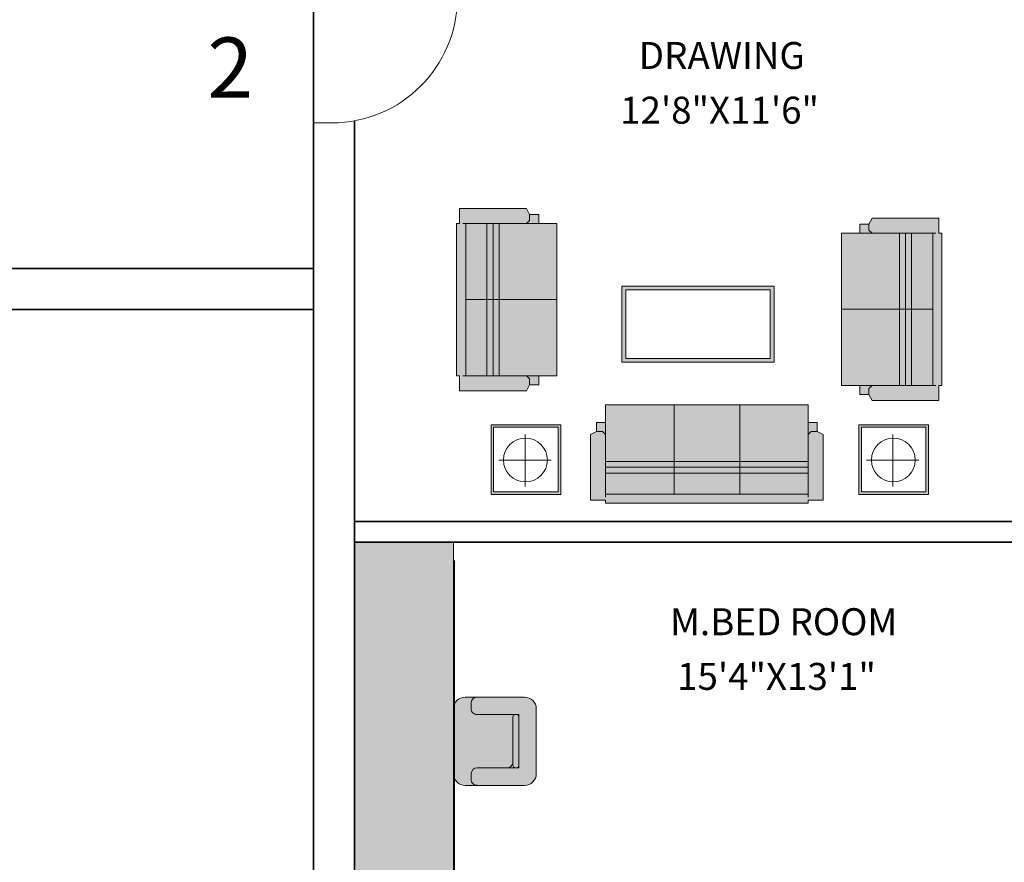
# Model space of a CAD drawing. Units: millimetres. Extents: x 27017497 to 27018854, y 7058029 to 7059154.
# Tile 78 of 91: x 27018246 to 27018462, y 7058224 to 7058409. Entities that reach past the tile are written whole.
import ezdxf

# ---------------------------------------------------------------- set-up
doc = ezdxf.new("R2010")
doc.units = ezdxf.units.MM
for name, color, linetype, lineweight in [('A-ANNO-DIMS', 2, 'Continuous', 18), ('A-ANNO-IDEN', 7, 'Continuous', 18), ('A-AREA-IDEN', 7, 'Continuous', 18), ('A-DOOR', 4, 'Continuous', 20), ('A-FLOR-CASE', 8, 'Continuous', 20), ('A-FLOR-CASE-PATT', 44, 'Continuous', 13), ('A-FURN', 8, 'Continuous', 18), ('A-WALL', 7, 'Continuous', 35)]:
    doc.layers.add(name, color=color, linetype=linetype, lineweight=lineweight)
doc.layers.add('A-FURN-PATT', color=177, linetype='Continuous', lineweight=13, true_color=0x293189)
doc.styles.get("Standard").update_dxf_attribs({"font": 'arial.ttf'})
doc.dimstyles.get("Standard").update_dxf_attribs({"dimtxt": 0.18, "dimasz": 0.18, "dimexe": 0.18, "dimexo": 0.0625, "dimgap": 0.09, "dimtad": 0, "dimtih": 1, "dimtoh": 1, "dimdec": 4, "dimzin": 0, "dimdsep": 46, "dimtxsty": 'Standard', "dimcen": 0.09, "dimadec": 0, "dimazin": 0, "dimtfac": 1, "dimtdec": 4, "dimtofl": 0, "dimtmove": 0, "dimatfit": 3, "dimfxl": 1, "dimtolj": 1, "dimtzin": 0, "dimarcsym": 0})

# ---------------------------------------------------------------- blocks, each defined once
blk = doc.blocks.new('*U2')
for p, q in [((0, 0), (0, -6)), ((40, 0), (40, -6))]:
    blk.add_line(p, q)
blk.add_lwpolyline([(0, 0), (0, 40), (1.75, 40), (1.75, 0)], close=True)
blk.add_arc((0, 0), 40, 0, 90)
blk = doc.blocks.new('CHAIR-OCCASIONAL')
for p, q in [((19.6, 18.74), (7.02, 22.21)), ((3.87, 20.42), (0.09, 6.71)), ((4.13, 6.92), (7.23, 18.17)), ((5.25, 10.97), (7.23, 18.17)), ((5.25, 10.97), (7.1, 17.68)), ((8.33, 17.34), (5.63, 7.52)), ((16.06, 15.73), (7.23, 18.17)), ((7.23, 18.17), (16.06, 15.73)), ((7.23, 18.17), (16.06, 15.73)), ((7.73, 18.03), (7.97, 17.97)), ((7.73, 18.03), (7.97, 17.97)), ((17.64, 16.63), (17.98, 17.86)), ((17.64, 16.63), (17.98, 17.86)), ((17.6, 1.88), (21.39, 15.6)), ((12.96, 4.48), (4.13, 6.92)), ((4.87, 6.71), (4.63, 6.78)), ((5.63, 7.52), (5.5, 7.07)), ((1.88, 3.56), (14.46, 0.09)), ((13.86, 2.91), (13.52, 1.68))]:
    blk.add_line(p, q)
for centre, radius, start, end in [((6.34, 19.74), 2.56, 74.5879, 164.5879), ((16.74, 18.2), 1.28, 344.5879, 74.5879), ((16.74, 18.2), 1.28, 344.5879, 74.5879), ((7.59, 17.54), 0.512, 74.5879, 164.5879), ((7.84, 17.47), 0.512, 344.5879, 74.5879), ((9.36, 16.26), 1.28, 74.5879, 164.5879), ((18.92, 16.28), 2.56, 344.5879, 74.5879), ((16.4, 16.97), 1.28, 254.5879, 344.5879), ((16.4, 16.97), 1.28, 254.5879, 344.5879), ((2.56, 6.03), 2.56, 164.5879, 254.5879), ((4.76, 7.28), 0.512, 164.5879, 254.5879), ((5.01, 7.21), 0.512, 254.5879, 344.5879), ((12.62, 3.25), 1.28, 344.5879, 74.5879), ((12.28, 2.02), 1.28, 254.5879, 344.5879), ((15.14, 2.56), 2.56, 254.5879, 344.5879)]:
    blk.add_arc(centre, radius, start, end)
blk = doc.blocks.new('SOFA-THREE-SEAT')
for p, q in [((47.73, 21.58), (3.27, 21.58)), ((3.27, 21.58), (3.27, 17.65)), ((18.31, 21.58), (18.31, 1.96)), ((32.69, 21.58), (32.69, 1.96)), ((47.73, 17.65), (47.73, 21.58)), ((3.27, 17.65), (1.31, 17.65)), ((1.31, 17.65), (1.31, 15.69)), ((3.27, 17.65), (3.27, 15.04)), ((47.73, 17.65), (47.73, 15.04)), ((49.69, 17.65), (47.73, 17.65)), ((49.69, 15.69), (49.69, 17.65)), ((1.31, 15.69), (0, 15.04)), ((1.31, 15.69), (2.62, 15.69)), ((2.62, 15.69), (3.27, 15.04)), ((48.38, 15.69), (47.73, 15.04)), ((49.69, 15.69), (48.38, 15.69)), ((51, 15.04), (49.69, 15.69)), ((0, 15.04), (0, 0.65)), ((3.27, 15.04), (3.27, 1.31)), ((47.73, 15.04), (47.73, 1.31)), ((51, 0.65), (51, 15.04)), ((47.73, 9.15), (3.27, 9.15)), ((47.73, 7.85), (3.27, 7.85)), ((47.73, 6.54), (3.27, 6.54)), ((0, 0.65), (3.27, 0.65)), ((3.27, 1.96), (47.73, 1.96)), ((3.27, 0.65), (3.27, 0)), ((47.73, 0), (47.73, 0.65)), ((47.73, 0.65), (51, 0.65)), ((3.27, 0), (47.73, 0))]:
    blk.add_line(p, q)
blk = doc.blocks.new('SETTEE-TWO-SEAT')
for p, q in [((6.67, 40.01), (6, 38.68)), ((21.34, 40.01), (6.67, 40.01)), ((21.34, 36.68), (21.34, 40.01)), ((6, 38.68), (4, 38.68)), ((4, 38.68), (4, 36.68)), ((6, 38.68), (6, 37.35)), ((6, 37.35), (6.67, 36.68)), ((0, 36.68), (0, 3.33)), ((4, 36.68), (0, 36.68)), ((4, 36.68), (6.67, 36.68)), ((6.67, 36.68), (20.67, 36.68)), ((12.67, 36.68), (12.67, 3.33)), ((14, 36.68), (14, 3.33)), ((15.34, 36.68), (15.34, 3.33)), ((20.01, 3.33), (20.01, 36.68)), ((22.01, 36.68), (21.34, 36.68)), ((22.01, 3.33), (22.01, 36.68)), ((0, 20.01), (20.01, 20.01)), ((0, 3.33), (4, 3.33)), ((4, 3.33), (6.67, 3.33)), ((4, 3.33), (4, 1.33)), ((6, 2.67), (6.67, 3.33)), ((6, 1.33), (6, 2.67)), ((6.67, 3.33), (20.67, 3.33)), ((21.34, 0), (21.34, 3.33)), ((21.34, 3.33), (22.01, 3.33)), ((4, 1.33), (6, 1.33)), ((6, 1.33), (6.67, 0)), ((6.67, 0), (21.34, 0))]:
    blk.add_line(p, q)
blk = doc.blocks.new('TABLE-END')
for p, q in [((15.28, 15.28), (0, 15.28)), ((0, 15.28), (0, 0)), ((15.28, 0), (15.28, 15.28)), ((14.73, 14.73), (0.56, 14.73)), ((0.56, 14.73), (0.56, 0.56)), ((7.79, 1.78), (7.79, 13.18)), ((14.73, 0.56), (14.73, 14.73)), ((2.12, 7.51), (13.57, 7.51)), ((0.56, 0.56), (14.73, 0.56)), ((0, 0), (15.28, 0))]:
    blk.add_line(p, q)
blk.add_circle((7.72, 7.57), 4.81)
blk = doc.blocks.new('TABLE-COFFEE')
for p, q in [((33.35, 16.67), (0, 16.67)), ((0, 16.67), (0, 0)), ((32.51, 15.84), (0.83, 15.84)), ((0.83, 15.84), (0.83, 0.83)), ((32.51, 0.83), (32.51, 15.84)), ((33.35, 0), (33.35, 16.67)), ((0, 0), (33.35, 0)), ((0.83, 0.83), (32.51, 0.83))]:
    blk.add_line(p, q)
blk = doc.blocks.new('*D47')
at = {"layer": 'A-ANNO-DIMS', "color": 0, "lineweight": -2, "transparency": 16777216}
for p, q in [((27017561.17, 7058294.35), (27017561.17, 7058028.6)), ((27018790.61, 7058294.35), (27018790.61, 7058028.6)), ((27017561.35, 7058028.78), (27018175.43, 7058028.78)), ((27018790.43, 7058028.78), (27018176.34, 7058028.78))]:
    blk.add_line(p, q, dxfattribs=at)
at = {"layer": 'A-ANNO-DIMS', "color": 0, "transparency": 16777216}
for points in [[(27017561.35, 7058028.81), (27017561.35, 7058028.75), (27017561.17, 7058028.78)], [(27018790.43, 7058028.81), (27018790.43, 7058028.75), (27018790.61, 7058028.78)]]:
    blk.add_solid(points, dxfattribs=at)
at = {"layer": 'Defpoints', "color": 0, "transparency": 16777216}
for p in [(27017561.17, 7058294.41), (27018790.61, 7058294.41), (27018790.61, 7058028.78)]:
    blk.add_point(p, dxfattribs=at)
at = {"layer": 'A-ANNO-DIMS', "color": 0, "transparency": 16777216, "insert": (27018175.89, 7058028.78), "char_height": 0.18, "attachment_point": 5}
blk.add_mtext('\\A1;1229.4', dxfattribs=at)
blk = doc.blocks.new('*D48')
at = {"layer": 'A-ANNO-DIMS', "color": 0, "lineweight": -2, "transparency": 16777216}
for p, q in [((27018463.5, 7058622.91), (27017497.54, 7058622.91)), ((27017497.72, 7058622.73), (27017497.72, 7058357.75)), ((27017497.72, 7058092.41), (27017497.72, 7058357.39)), ((27018555.13, 7058092.23), (27017497.54, 7058092.23))]:
    blk.add_line(p, q, dxfattribs=at)
at = {"layer": 'A-ANNO-DIMS', "color": 0, "transparency": 16777216}
for points in [[(27017497.69, 7058622.73), (27017497.75, 7058622.73), (27017497.72, 7058622.91)], [(27017497.69, 7058092.41), (27017497.75, 7058092.41), (27017497.72, 7058092.23)]]:
    blk.add_solid(points, dxfattribs=at)
at = {"layer": 'Defpoints', "color": 0, "transparency": 16777216}
for p in [(27018463.56, 7058622.91), (27017497.72, 7058092.23), (27018555.19, 7058092.23)]:
    blk.add_point(p, dxfattribs=at)
at = {"layer": 'A-ANNO-DIMS', "color": 0, "transparency": 16777216, "insert": (27017497.72, 7058357.57), "char_height": 0.18, "attachment_point": 5}
blk.add_mtext('\\A1;530.7', dxfattribs=at)
blk = doc.blocks.new('*D51')
at = {"layer": 'A-ANNO-DIMS', "color": 0, "lineweight": -2, "transparency": 16777216}
for p, q in [((27018041.17, 7058345.35), (27018041.17, 7058028.6)), ((27018310.61, 7058345.35), (27018310.61, 7058028.6)), ((27018041.35, 7058028.78), (27018175.42, 7058028.78)), ((27018310.43, 7058028.78), (27018176.35, 7058028.78))]:
    blk.add_line(p, q, dxfattribs=at)
at = {"layer": 'A-ANNO-DIMS', "color": 0, "transparency": 16777216}
for points in [[(27018041.35, 7058028.81), (27018041.35, 7058028.75), (27018041.17, 7058028.78)], [(27018310.43, 7058028.81), (27018310.43, 7058028.75), (27018310.61, 7058028.78)]]:
    blk.add_solid(points, dxfattribs=at)
at = {"layer": 'Defpoints', "color": 0, "transparency": 16777216}
for p in [(27018041.17, 7058345.41), (27018310.61, 7058345.41), (27018310.61, 7058028.78)]:
    blk.add_point(p, dxfattribs=at)
at = {"layer": 'A-ANNO-DIMS', "color": 0, "transparency": 16777216, "insert": (27018175.89, 7058028.78), "char_height": 0.18, "attachment_point": 5}
blk.add_mtext('\\A1;269.44', dxfattribs=at)

msp = doc.modelspace()

# ---------------------------------------------------------------- hatches: boundary and pattern name
at = {"layer": 'A-FLOR-CASE-PATT'}
h = msp.add_hatch(color=256, dxfattribs=at)
h.dxf.hatch_style = 1
edge = h.paths.add_edge_path()
edge.add_line((27018341.343, 7058207.055), (27018330.837, 7058207.055))
edge.add_line((27018330.837, 7058207.055), (27018330.837, 7058203.02))
edge.add_line((27018330.837, 7058203.02), (27018338.424, 7058203.02))
edge.add_ellipse((27018338.23, 7058202.551), major_axis=(0.528, 0), ratio=0.8888917, start_angle=0, end_angle=90, ccw=False)
edge.add_line((27018338.758, 7058202.551), (27018338.758, 7058202.238))
edge.add_line((27018338.758, 7058202.238), (27018330.837, 7058201.488))
edge.add_line((27018330.837, 7058201.488), (27018330.837, 7058199.747))
edge.add_line((27018330.837, 7058199.747), (27018338.424, 7058199.747))
edge.add_ellipse((27018338.23, 7058199.277), major_axis=(0.528, 0), ratio=0.8888917, start_angle=0, end_angle=90, ccw=False)
edge.add_line((27018338.758, 7058199.277), (27018338.758, 7058198.964))
edge.add_line((27018338.758, 7058198.964), (27018330.837, 7058198.215))
edge.add_line((27018330.837, 7058198.215), (27018330.837, 7058193.415))
edge.add_line((27018330.837, 7058193.415), (27018338.284, 7058190.704))
edge.add_ellipse((27018337.942, 7058190.329), major_axis=(0.496, -0.181), ratio=0.8888917, start_angle=0, end_angle=90, ccw=False)
edge.add_line((27018338.439, 7058190.148), (27018338.331, 7058189.854))
edge.add_line((27018338.331, 7058189.854), (27018330.837, 7058191.806))
edge.add_line((27018330.837, 7058191.806), (27018330.837, 7058188.22))
edge.add_line((27018330.837, 7058188.22), (27018338.424, 7058188.22))
edge.add_ellipse((27018338.23, 7058187.75), major_axis=(0.528, 0), ratio=0.8888917, start_angle=0, end_angle=90, ccw=False)
edge.add_line((27018338.758, 7058187.75), (27018338.758, 7058187.437))
edge.add_line((27018338.758, 7058187.437), (27018330.837, 7058186.688))
edge.add_line((27018330.837, 7058186.688), (27018330.837, 7058181.982))
edge.add_line((27018330.837, 7058181.982), (27018338.424, 7058181.982))
edge.add_ellipse((27018338.23, 7058181.513), major_axis=(0.528, 0), ratio=0.8888917, start_angle=0, end_angle=90, ccw=False)
edge.add_line((27018338.758, 7058181.513), (27018338.758, 7058181.199))
edge.add_line((27018338.758, 7058181.199), (27018330.837, 7058180.45))
edge.add_line((27018330.837, 7058180.45), (27018330.837, 7058178.709))
edge.add_line((27018330.837, 7058178.709), (27018338.424, 7058178.709))
edge.add_ellipse((27018338.23, 7058178.239), major_axis=(0.528, 0), ratio=0.8888917, start_angle=0, end_angle=90, ccw=False)
edge.add_line((27018338.758, 7058178.239), (27018338.758, 7058177.926))
edge.add_line((27018338.758, 7058177.926), (27018330.837, 7058177.177))
edge.add_line((27018330.837, 7058177.177), (27018330.837, 7058173.878))
edge.add_line((27018330.837, 7058173.878), (27018338.284, 7058171.167))
edge.add_ellipse((27018337.942, 7058170.792), major_axis=(0.496, -0.181), ratio=0.8888917, start_angle=0, end_angle=90, ccw=False)
edge.add_line((27018338.439, 7058170.611), (27018338.331, 7058170.317))
edge.add_line((27018338.331, 7058170.317), (27018330.837, 7058172.269))
edge.add_line((27018330.837, 7058172.269), (27018330.837, 7058168.293))
edge.add_line((27018330.837, 7058168.293), (27018338.424, 7058168.293))
edge.add_ellipse((27018338.23, 7058167.824), major_axis=(0.528, 0), ratio=0.8888917, start_angle=0, end_angle=90, ccw=False)
edge.add_line((27018338.758, 7058167.824), (27018338.758, 7058167.511))
edge.add_line((27018338.758, 7058167.511), (27018330.837, 7058166.762))
edge.add_line((27018330.837, 7058166.762), (27018330.837, 7058160.389))
edge.add_line((27018330.837, 7058160.389), (27018338.424, 7058160.389))
edge.add_ellipse((27018338.23, 7058159.92), major_axis=(0.528, 0), ratio=0.8888917, start_angle=0, end_angle=90, ccw=False)
edge.add_line((27018338.758, 7058159.92), (27018338.758, 7058159.607))
edge.add_line((27018338.758, 7058159.607), (27018330.837, 7058158.858))
edge.add_line((27018330.837, 7058158.858), (27018330.837, 7058157.116))
edge.add_line((27018330.837, 7058157.116), (27018338.424, 7058157.116))
edge.add_ellipse((27018338.23, 7058156.647), major_axis=(0.528, 0), ratio=0.8888917, start_angle=0, end_angle=90, ccw=False)
edge.add_line((27018338.758, 7058156.647), (27018338.758, 7058156.334))
edge.add_line((27018338.758, 7058156.334), (27018330.837, 7058155.585))
edge.add_line((27018330.837, 7058155.585), (27018330.837, 7058150.784))
edge.add_line((27018330.837, 7058150.784), (27018338.284, 7058148.073))
edge.add_ellipse((27018337.942, 7058147.698), major_axis=(0.496, -0.181), ratio=0.8888917, start_angle=0, end_angle=90, ccw=False)
edge.add_line((27018338.439, 7058147.517), (27018338.331, 7058147.223))
edge.add_line((27018338.331, 7058147.223), (27018330.837, 7058149.175))
edge.add_line((27018330.837, 7058149.175), (27018330.837, 7058145.589))
edge.add_line((27018330.837, 7058145.589), (27018338.424, 7058145.589))
edge.add_ellipse((27018338.23, 7058145.119), major_axis=(0.528, 0), ratio=0.8888917, start_angle=0, end_angle=90, ccw=False)
edge.add_line((27018338.758, 7058145.119), (27018338.758, 7058144.806))
edge.add_line((27018338.758, 7058144.806), (27018330.837, 7058144.057))
edge.add_line((27018330.837, 7058144.057), (27018330.837, 7058141.912))
edge.add_line((27018330.837, 7058141.912), (27018341.343, 7058141.912))
edge.add_line((27018341.343, 7058141.912), (27018341.343, 7058207.055))
edge = h.paths.add_edge_path()
edge.add_line((27018330.112, 7058207.055), (27018319.606, 7058207.055))
edge.add_line((27018319.606, 7058207.055), (27018319.606, 7058141.912))
edge.add_line((27018319.606, 7058141.912), (27018330.112, 7058141.912))
edge.add_line((27018330.112, 7058141.912), (27018330.112, 7058144.024))
edge.add_line((27018330.112, 7058144.024), (27018322.543, 7058144.024))
edge.add_ellipse((27018322.736, 7058144.493), major_axis=(0.528, 0), ratio=0.8888917, start_angle=180, end_angle=270, ccw=False)
edge.add_line((27018322.208, 7058144.493), (27018322.208, 7058145.291))
edge.add_ellipse((27018322.736, 7058145.119), major_axis=(0.528, 0), ratio=0.8888917, start_angle=90, end_angle=180, ccw=False)
edge.add_line((27018322.736, 7058145.589), (27018330.112, 7058145.589))
edge.add_line((27018330.112, 7058145.589), (27018330.112, 7058149.382))
edge.add_line((27018330.112, 7058149.382), (27018322.826, 7058152.034))
edge.add_ellipse((27018323.168, 7058152.409), major_axis=(0.496, -0.181), ratio=0.8888917, start_angle=180, end_angle=270, ccw=False)
edge.add_line((27018322.672, 7058152.59), (27018322.945, 7058153.34))
edge.add_ellipse((27018323.382, 7058152.997), major_axis=(0.496, -0.181), ratio=0.8888917, start_angle=90, end_angle=180, ccw=False)
edge.add_line((27018323.543, 7058153.439), (27018330.112, 7058151.048))
edge.add_line((27018330.112, 7058151.048), (27018330.112, 7058155.551))
edge.add_line((27018330.112, 7058155.551), (27018322.543, 7058155.551))
edge.add_ellipse((27018322.736, 7058156.021), major_axis=(0.528, 0), ratio=0.8888917, start_angle=180, end_angle=270, ccw=False)
edge.add_line((27018322.208, 7058156.021), (27018322.208, 7058156.819))
edge.add_ellipse((27018322.736, 7058156.647), major_axis=(0.528, 0), ratio=0.8888917, start_angle=90, end_angle=180, ccw=False)
edge.add_line((27018322.736, 7058157.116), (27018330.112, 7058157.116))
edge.add_line((27018330.112, 7058157.116), (27018330.112, 7058158.824))
edge.add_line((27018330.112, 7058158.824), (27018322.543, 7058158.824))
edge.add_ellipse((27018322.736, 7058159.294), major_axis=(0.528, 0), ratio=0.8888917, start_angle=180, end_angle=270, ccw=False)
edge.add_line((27018322.208, 7058159.294), (27018322.208, 7058160.092))
edge.add_ellipse((27018322.736, 7058159.92), major_axis=(0.528, 0), ratio=0.8888917, start_angle=90, end_angle=180, ccw=False)
edge.add_line((27018322.736, 7058160.389), (27018330.112, 7058160.389))
edge.add_line((27018330.112, 7058160.389), (27018330.112, 7058166.728))
edge.add_line((27018330.112, 7058166.728), (27018322.543, 7058166.728))
edge.add_ellipse((27018322.736, 7058167.198), major_axis=(0.528, 0), ratio=0.8888917, start_angle=180, end_angle=270, ccw=False)
edge.add_line((27018322.208, 7058167.198), (27018322.208, 7058167.996))
edge.add_ellipse((27018322.736, 7058167.824), major_axis=(0.528, 0), ratio=0.8888917, start_angle=90, end_angle=180, ccw=False)
edge.add_line((27018322.736, 7058168.293), (27018330.112, 7058168.293))
edge.add_line((27018330.112, 7058168.293), (27018330.112, 7058172.476))
edge.add_line((27018330.112, 7058172.476), (27018322.826, 7058175.128))
edge.add_ellipse((27018323.168, 7058175.503), major_axis=(0.496, -0.181), ratio=0.8888917, start_angle=180, end_angle=270, ccw=False)
edge.add_line((27018322.672, 7058175.684), (27018322.945, 7058176.433))
edge.add_ellipse((27018323.382, 7058176.091), major_axis=(0.496, -0.181), ratio=0.8888917, start_angle=90, end_angle=180, ccw=False)
edge.add_line((27018323.543, 7058176.533), (27018330.112, 7058174.142))
edge.add_line((27018330.112, 7058174.142), (27018330.112, 7058177.144))
edge.add_line((27018330.112, 7058177.144), (27018322.543, 7058177.144))
edge.add_ellipse((27018322.736, 7058177.613), major_axis=(0.528, 0), ratio=0.8888917, start_angle=180, end_angle=270, ccw=False)
edge.add_line((27018322.208, 7058177.613), (27018322.208, 7058178.411))
edge.add_ellipse((27018322.736, 7058178.239), major_axis=(0.528, 0), ratio=0.8888917, start_angle=90, end_angle=180, ccw=False)
edge.add_line((27018322.736, 7058178.709), (27018330.112, 7058178.709))
edge.add_line((27018330.112, 7058178.709), (27018330.112, 7058180.417))
edge.add_line((27018330.112, 7058180.417), (27018322.543, 7058180.417))
edge.add_ellipse((27018322.736, 7058180.886), major_axis=(0.528, 0), ratio=0.8888917, start_angle=180, end_angle=270, ccw=False)
edge.add_line((27018322.208, 7058180.886), (27018322.208, 7058181.684))
edge.add_ellipse((27018322.736, 7058181.513), major_axis=(0.528, 0), ratio=0.8888917, start_angle=90, end_angle=180, ccw=False)
edge.add_line((27018322.736, 7058181.982), (27018330.112, 7058181.982))
edge.add_line((27018330.112, 7058181.982), (27018330.112, 7058186.655))
edge.add_line((27018330.112, 7058186.655), (27018322.543, 7058186.655))
edge.add_ellipse((27018322.736, 7058187.124), major_axis=(0.528, 0), ratio=0.8888917, start_angle=180, end_angle=270, ccw=False)
edge.add_line((27018322.208, 7058187.124), (27018322.208, 7058187.922))
edge.add_ellipse((27018322.736, 7058187.75), major_axis=(0.528, 0), ratio=0.8888917, start_angle=90, end_angle=180, ccw=False)
edge.add_line((27018322.736, 7058188.22), (27018330.112, 7058188.22))
edge.add_line((27018330.112, 7058188.22), (27018330.112, 7058192.013))
edge.add_line((27018330.112, 7058192.013), (27018322.826, 7058194.665))
edge.add_ellipse((27018323.168, 7058195.04), major_axis=(0.496, -0.181), ratio=0.8888917, start_angle=180, end_angle=270, ccw=False)
edge.add_line((27018322.672, 7058195.22), (27018322.945, 7058195.97))
edge.add_ellipse((27018323.382, 7058195.628), major_axis=(0.496, -0.181), ratio=0.8888917, start_angle=90, end_angle=180, ccw=False)
edge.add_line((27018323.543, 7058196.069), (27018330.112, 7058193.678))
edge.add_line((27018330.112, 7058193.678), (27018330.112, 7058198.182))
edge.add_line((27018330.112, 7058198.182), (27018322.543, 7058198.182))
edge.add_ellipse((27018322.736, 7058198.651), major_axis=(0.528, 0), ratio=0.8888917, start_angle=180, end_angle=270, ccw=False)
edge.add_line((27018322.208, 7058198.651), (27018322.208, 7058199.449))
edge.add_ellipse((27018322.736, 7058199.277), major_axis=(0.528, 0), ratio=0.8888917, start_angle=90, end_angle=180, ccw=False)
edge.add_line((27018322.736, 7058199.747), (27018330.112, 7058199.747))
edge.add_line((27018330.112, 7058199.747), (27018330.112, 7058201.455))
edge.add_line((27018330.112, 7058201.455), (27018322.543, 7058201.455))
edge.add_ellipse((27018322.736, 7058201.924), major_axis=(0.528, 0), ratio=0.8888917, start_angle=180, end_angle=270, ccw=False)
edge.add_line((27018322.208, 7058201.924), (27018322.208, 7058202.722))
edge.add_ellipse((27018322.736, 7058202.551), major_axis=(0.528, 0), ratio=0.8888917, start_angle=90, end_angle=180, ccw=False)
edge.add_line((27018322.736, 7058203.02), (27018330.112, 7058203.02))
edge.add_line((27018330.112, 7058203.02), (27018330.112, 7058207.055))
h.paths.add_polyline_path([(27018341.31, 7058294.412), (27018319.606, 7058294.412), (27018319.606, 7058207.1), (27018341.31, 7058207.1)])
h.paths.add_polyline_path([(27018354.358, 7058255.592), (27018354.358, 7058256.057, -0.4142136), (27018354.869, 7058256.569), (27018346.477, 7058256.569, -0.4142136), (27018345.197, 7058257.848), (27018345.197, 7058259.128, -0.4142136), (27018346.477, 7058260.407), (27018343.868, 7058260.407, 0.2909788), (27018341.551, 7058258.934), (27018341.551, 7058242.534, 0.2909788), (27018343.868, 7058241.06), (27018346.477, 7058241.06, -0.4142136), (27018345.197, 7058242.34), (27018345.197, 7058243.619, -0.4142136), (27018346.477, 7058244.899), (27018353.078, 7058244.899, 0.4142136), (27018354.358, 7058246.178)])
h.paths.add_polyline_path([(27018356.917, 7058260.407), (27018346.477, 7058260.407, 0.4142136), (27018345.197, 7058259.128), (27018345.197, 7058257.848, 0.4142136), (27018346.477, 7058256.569), (27018355.637, 7058256.569), (27018355.637, 7058244.899), (27018346.477, 7058244.899, 0.4142136), (27018345.197, 7058243.619), (27018345.197, 7058242.34, 0.4142136), (27018346.477, 7058241.06), (27018356.917, 7058241.06, 0.4142136), (27018359.476, 7058243.619), (27018359.476, 7058257.848, 0.4142136)])
h.paths.add_polyline_path([(27018355.637, 7058252.362), (27018355.637, 7058256.057, 0.4903144), (27018354.997, 7058256.553, 0.4903144), (27018354.358, 7058256.057), (27018354.358, 7058255.592), (27018354.358, 7058245.411, 0.4903144), (27018354.997, 7058244.915, 0.4903144), (27018355.637, 7058245.411)], flags=17)
at = {"layer": 'A-FURN-PATT'}
h = msp.add_hatch(color=256, dxfattribs=at)
h.dxf.hatch_style = 1
h.paths.add_polyline_path([(27018364.003, 7058364.252), (27018360.002, 7058364.252), (27018357.334, 7058364.252), (27018351.332, 7058364.252), (27018351.332, 7058347.58), (27018364.003, 7058347.58)])
h.paths.add_polyline_path([(27018364.003, 7058347.58), (27018351.332, 7058347.58), (27018351.332, 7058330.907), (27018357.334, 7058330.907), (27018360.002, 7058330.907), (27018364.003, 7058330.907)])
h.paths.add_polyline_path([(27018348.664, 7058347.58), (27018343.996, 7058347.58), (27018343.996, 7058330.907), (27018348.664, 7058330.907)], flags=17)
h.paths.add_polyline_path([(27018348.664, 7058364.252), (27018343.996, 7058364.252), (27018343.996, 7058347.58), (27018348.664, 7058347.58)], flags=17)
h.paths.add_polyline_path([(27018343.996, 7058364.252), (27018357.334, 7058364.252), (27018358.001, 7058364.919), (27018358.001, 7058366.253), (27018357.334, 7058367.587), (27018342.662, 7058367.587), (27018342.662, 7058364.252), (27018341.995, 7058364.252), (27018341.995, 7058330.907), (27018342.662, 7058330.907), (27018342.662, 7058327.573), (27018357.334, 7058327.573), (27018358.001, 7058328.907), (27018358.001, 7058330.241), (27018357.334, 7058330.907), (27018343.996, 7058330.907)])
h.paths.add_polyline_path([(27018349.998, 7058364.252), (27018348.664, 7058364.252), (27018348.664, 7058347.58), (27018349.998, 7058347.58)], flags=17)
h.paths.add_polyline_path([(27018351.332, 7058364.252), (27018349.998, 7058364.252), (27018349.998, 7058347.58), (27018351.332, 7058347.58)], flags=17)
h.paths.add_polyline_path([(27018349.998, 7058347.58), (27018348.664, 7058347.58), (27018348.664, 7058330.907), (27018349.998, 7058330.907)], flags=17)
h.paths.add_polyline_path([(27018351.332, 7058347.58), (27018349.998, 7058347.58), (27018349.998, 7058330.907), (27018351.332, 7058330.907)], flags=17)
h.paths.add_polyline_path([(27018360.002, 7058330.907), (27018357.334, 7058330.907), (27018358.001, 7058330.241), (27018358.001, 7058328.907), (27018360.002, 7058328.907)])
h.paths.add_polyline_path([(27018360.002, 7058366.253), (27018358.001, 7058366.253), (27018358.001, 7058364.919), (27018357.334, 7058364.252), (27018360.002, 7058364.252)])
h.paths.add_polyline_path([(27018411.612, 7058350.536), (27018378.268, 7058350.536), (27018378.268, 7058333.863), (27018411.612, 7058333.863)])
h.paths.add_polyline_path([(27018410.779, 7058349.702), (27018410.779, 7058334.697), (27018379.101, 7058334.697), (27018379.101, 7058349.702)], flags=16)
h = msp.add_hatch(color=256, dxfattribs=at)
h.dxf.hatch_style = 1
h.paths.add_polyline_path([(27018439.111, 7058362.129), (27018433.109, 7058362.129), (27018430.441, 7058362.129), (27018426.44, 7058362.129), (27018426.44, 7058345.456), (27018439.111, 7058345.456)])
h.paths.add_polyline_path([(27018439.111, 7058345.456), (27018426.44, 7058345.456), (27018426.44, 7058328.784), (27018430.441, 7058328.784), (27018433.109, 7058328.784), (27018439.111, 7058328.784)])
h.paths.add_polyline_path([(27018446.446, 7058362.129), (27018441.778, 7058362.129), (27018441.778, 7058345.456), (27018446.446, 7058345.456)], flags=17)
h.paths.add_polyline_path([(27018446.446, 7058345.456), (27018441.778, 7058345.456), (27018441.778, 7058328.784), (27018446.446, 7058328.784)], flags=17)
h.paths.add_polyline_path([(27018440.444, 7058345.456), (27018439.111, 7058345.456), (27018439.111, 7058328.784), (27018440.444, 7058328.784)], flags=17)
h.paths.add_polyline_path([(27018441.778, 7058345.456), (27018440.444, 7058345.456), (27018440.444, 7058328.784), (27018441.778, 7058328.784)], flags=17)
h.paths.add_polyline_path([(27018441.778, 7058362.129), (27018440.444, 7058362.129), (27018440.444, 7058345.456), (27018441.778, 7058345.456)], flags=17)
h.paths.add_polyline_path([(27018440.444, 7058362.129), (27018439.111, 7058362.129), (27018439.111, 7058345.456), (27018440.444, 7058345.456)], flags=17)
h.paths.add_polyline_path([(27018447.78, 7058365.463), (27018433.109, 7058365.463), (27018432.442, 7058364.13), (27018432.442, 7058362.796), (27018433.109, 7058362.129), (27018446.446, 7058362.129), (27018446.446, 7058328.784), (27018433.109, 7058328.784), (27018432.442, 7058328.117), (27018432.442, 7058326.783), (27018433.109, 7058325.45), (27018447.78, 7058325.45), (27018447.78, 7058328.784), (27018448.447, 7058328.784), (27018448.447, 7058362.129), (27018447.78, 7058362.129)])
h.paths.add_polyline_path([(27018432.442, 7058364.13), (27018430.441, 7058364.13), (27018430.441, 7058362.129), (27018433.109, 7058362.129), (27018432.442, 7058362.796)])
h.paths.add_polyline_path([(27018432.442, 7058328.117), (27018433.109, 7058328.784), (27018430.441, 7058328.784), (27018430.441, 7058326.783), (27018432.442, 7058326.783)])
h = msp.add_hatch(color=256, dxfattribs=at)
h.dxf.hatch_style = 1
h.paths.add_polyline_path([(27018419.12, 7058317.992), (27018419.12, 7058320.608), (27018419.12, 7058324.531), (27018404.083, 7058324.531), (27018404.083, 7058312.108), (27018419.12, 7058312.108)])
h.paths.add_polyline_path([(27018419.12, 7058309.493), (27018404.083, 7058309.493), (27018404.083, 7058304.916), (27018419.12, 7058304.916)], flags=17)
h.paths.add_polyline_path([(27018404.083, 7058324.531), (27018389.699, 7058324.531), (27018389.699, 7058312.108), (27018404.083, 7058312.108)])
h.paths.add_polyline_path([(27018389.699, 7058324.531), (27018374.661, 7058324.531), (27018374.661, 7058320.608), (27018374.661, 7058317.992), (27018374.661, 7058312.108), (27018389.699, 7058312.108)])
h.paths.add_polyline_path([(27018374.661, 7058317.992), (27018374.007, 7058318.646), (27018372.699, 7058318.646), (27018371.392, 7058317.992), (27018371.392, 7058303.608), (27018374.661, 7058303.608), (27018374.661, 7058302.955), (27018419.12, 7058302.955), (27018419.12, 7058303.608), (27018422.39, 7058303.608), (27018422.39, 7058317.992), (27018421.082, 7058318.646), (27018419.774, 7058318.646), (27018419.12, 7058317.992), (27018419.12, 7058312.108), (27018419.12, 7058304.916), (27018404.083, 7058304.916), (27018374.661, 7058304.916)])
h.paths.add_polyline_path([(27018389.699, 7058309.493), (27018374.661, 7058309.493), (27018374.661, 7058304.916), (27018389.699, 7058304.916)], flags=17)
h.paths.add_polyline_path([(27018404.083, 7058309.493), (27018389.699, 7058309.493), (27018389.699, 7058304.916), (27018404.083, 7058304.916)], flags=17)
h.paths.add_polyline_path([(27018419.12, 7058312.108), (27018404.083, 7058312.108), (27018404.083, 7058310.8), (27018419.12, 7058310.8)], flags=17)
h.paths.add_polyline_path([(27018404.083, 7058312.108), (27018389.699, 7058312.108), (27018389.699, 7058310.8), (27018404.083, 7058310.8)], flags=17)
h.paths.add_polyline_path([(27018389.699, 7058312.108), (27018374.661, 7058312.108), (27018374.661, 7058310.8), (27018389.699, 7058310.8)], flags=17)
h.paths.add_polyline_path([(27018389.699, 7058310.8), (27018374.661, 7058310.8), (27018374.661, 7058309.493), (27018389.699, 7058309.493)], flags=17)
h.paths.add_polyline_path([(27018404.083, 7058310.8), (27018389.699, 7058310.8), (27018389.699, 7058309.493), (27018404.083, 7058309.493)], flags=17)
h.paths.add_polyline_path([(27018419.12, 7058310.8), (27018404.083, 7058310.8), (27018404.083, 7058309.493), (27018419.12, 7058309.493)], flags=17)
h.paths.add_polyline_path([(27018421.082, 7058320.608), (27018419.12, 7058320.608), (27018419.12, 7058317.992), (27018419.774, 7058318.646), (27018421.082, 7058318.646)])
h.paths.add_polyline_path([(27018374.661, 7058320.608), (27018372.699, 7058320.608), (27018372.699, 7058318.646), (27018374.007, 7058318.646), (27018374.661, 7058317.992)])
h = msp.add_hatch(color=256, dxfattribs=at)
h.dxf.hatch_style = 1
h.paths.add_polyline_path([(27018364.823, 7058320.14), (27018349.54, 7058320.14), (27018349.54, 7058304.857), (27018364.823, 7058304.857)])
h.paths.add_polyline_path([(27018364.268, 7058319.584), (27018364.268, 7058305.412), (27018350.096, 7058305.412), (27018350.096, 7058319.584)], flags=16)
h.paths.add_polyline_path([(27018361.909, 7058312.427, -1), (27018352.288, 7058312.427, -1)], flags=0)
h = msp.add_hatch(color=256, dxfattribs=at)
h.dxf.hatch_style = 1
h.paths.add_polyline_path([(27018445.496, 7058320.14), (27018430.213, 7058320.14), (27018430.213, 7058304.857), (27018445.496, 7058304.857)])
h.paths.add_polyline_path([(27018444.94, 7058319.584), (27018444.94, 7058305.412), (27018430.769, 7058305.412), (27018430.769, 7058319.584)], flags=16)
h.paths.add_polyline_path([(27018442.582, 7058312.427, -1), (27018432.961, 7058312.427, -1)], flags=0)

# ---------------------------------------------------------------- linework, layer by layer
at = {"layer": 'A-FLOR-CASE'}
for p, q in [((27018341.31, 7058207.055), (27018341.31, 7058294.412)), ((27018341.551, 7058290.392), (27018341.551, 7058203.035)), ((27018319.573, 7058207.055), (27018319.573, 7058251.237))]:
    msp.add_line(p, q, dxfattribs=at)
at = {"layer": 'A-WALL'}
for p, q in [((27018310.606, 7058589.912), (27018310.606, 7058169.223)), ((27018319.606, 7058386.803), (27018319.606, 7058141.912)), ((27018310.606, 7058386.357), (27018310.606, 7058375.363)), ((27018310.606, 7058386.357), (27018310.606, 7058246.045)), ((27018310.606, 7058386.357), (27018310.606, 7058132.912)), ((27018041.166, 7058354.412), (27018310.606, 7058354.412)), ((27018041.166, 7058345.412), (27018310.606, 7058345.412)), ((27018545.106, 7058298.912), (27018319.606, 7058298.912)), ((27018549.606, 7058294.412), (27018319.606, 7058294.412))]:
    msp.add_line(p, q, dxfattribs=at)
msp.add_lwpolyline([(27018319.594, 7058237.363), (27018319.594, 7058375.363)], dxfattribs=at)

# ---------------------------------------------------------------- block references
at = {"layer": 'A-DOOR', "xscale": 0.6870473523349573, "yscale": 0.6870473523349573, "zscale": 0.6870473523349573, "rotation": 270}
msp.add_blockref('*U2', (27018314.676, 7058413.839), dxfattribs=at)
at = {"layer": 'A-FURN', "extrusion": (0, 0, -1), "zscale": -1}
for name, p in [('SETTEE-TWO-SEAT', (-27018364.003, 7058327.573)), ('TABLE-COFFEE', (-27018411.613, 7058333.863)), ('SOFA-THREE-SEAT', (-27018422.39, 7058302.955)), ('TABLE-END', (-27018364.823, 7058304.857)), ('TABLE-END', (-27018445.496, 7058304.857))]:
    msp.add_blockref(name, p, dxfattribs=at)
at = {"layer": 'A-FURN'}
msp.add_blockref('SETTEE-TWO-SEAT', (27018426.44, 7058325.45), dxfattribs=at)
at = {"layer": 'A-FURN', "rotation": 195.4121391531662}
msp.add_blockref('CHAIR-OCCASIONAL', (27018357.782, 7058264.337), dxfattribs=at)

# ---------------------------------------------------------------- texts
at = {"layer": 'A-ANNO-DIMS'}
for s, p in [('12\'8"X11\'6"', (27018377.859, 7058386.175)), ('15\'4"X13\'1"', (27018390.351, 7058261.993))]:
    msp.add_text(s, height=5.91176, dxfattribs=at).set_placement(p)
at = {"layer": 'A-ANNO-IDEN'}
msp.add_text('2', height=13.242, dxfattribs=at).set_placement((27018287.324, 7058391.843))
at = {"layer": 'A-AREA-IDEN'}
for s, p in [('DRAWING', (27018381.954, 7058398.172)), ('M.BED ROOM', (27018388.816, 7058273.991))]:
    msp.add_text(s, height=5.9118, dxfattribs=at).set_placement(p)

# ---------------------------------------------------------------- dimensions: what is measured, and where the dimension line sits
at = {"layer": 'A-ANNO-DIMS'}
dim = msp.add_linear_dim(base=(27017497.716, 7058092.23), p1=(27018463.561, 7058622.912), p2=(27018555.192, 7058092.23), angle=90, dimstyle='Standard', override={"dimdec": 1, "dimlfac": 1, "dimrnd": 0, "dimzin": 0, "dimdsep": 46, "dimlunit": 2}, dxfattribs=at)
dim.commit()
dim.dimension.update_dxf_attribs({"geometry": '*D48', "text_midpoint": (27017497.716, 7058357.571)})
for base, p1, p2, override, picture in [((27018310.606, 7058028.78), (27018041.166, 7058345.412), (27018310.606, 7058345.412), {"dimdec": 2, "dimlfac": 1, "dimrnd": 0, "dimzin": 0, "dimdsep": 46, "dimlunit": 2}, '*D51'), ((27018790.606, 7058028.78), (27017561.166, 7058294.412), (27018790.606, 7058294.412), {"dimdec": 1, "dimlfac": 1, "dimrnd": 0, "dimzin": 0, "dimdsep": 46, "dimlunit": 2}, '*D47')]:
    dim = msp.add_linear_dim(base=base, p1=p1, p2=p2, dimstyle='Standard', override=override, dxfattribs=at)
    dim.commit()
    dim.dimension.update_dxf_attribs({"geometry": picture, "text_midpoint": (27018175.886, 7058028.78)})

doc.saveas('drawing.dxf')
